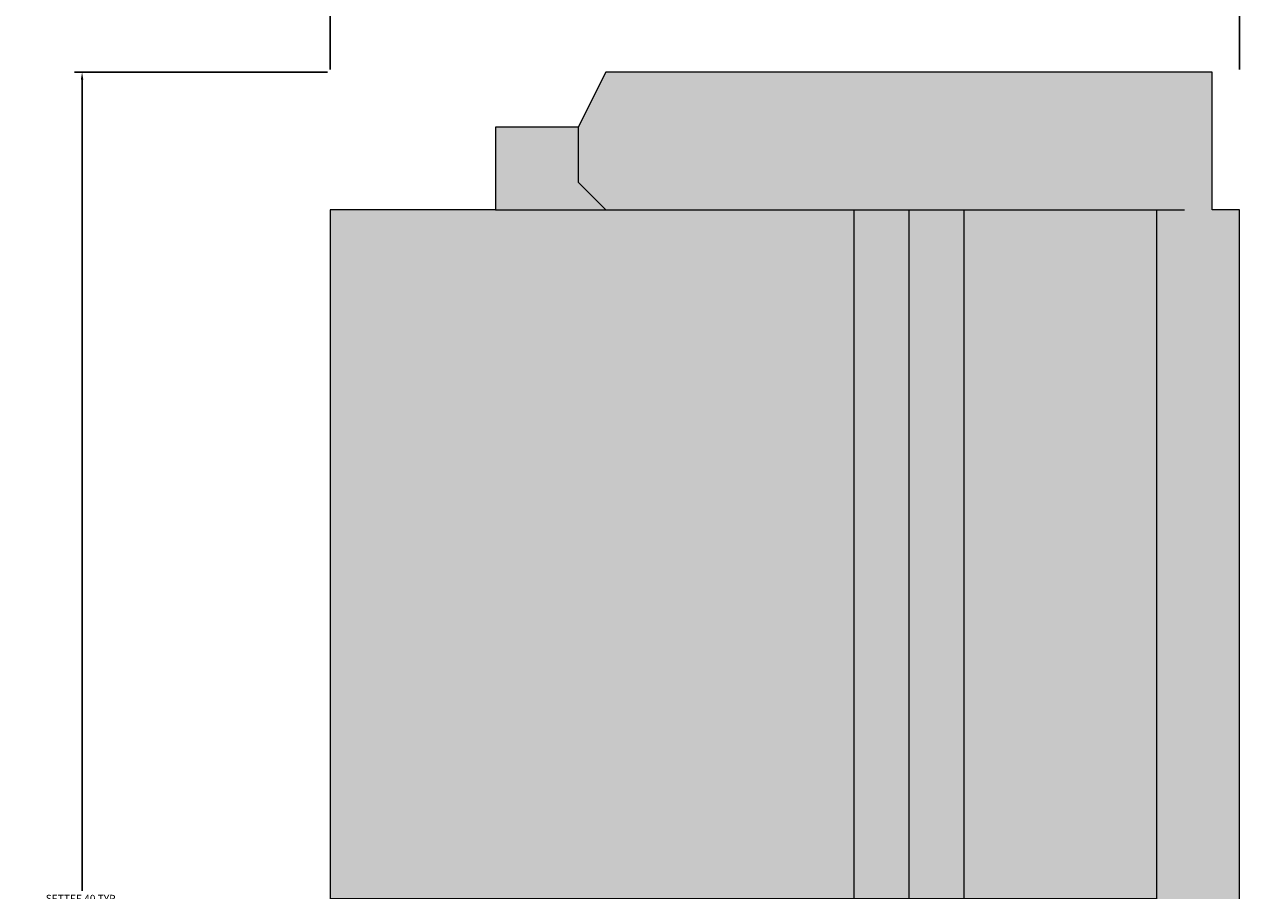
# Model space of a CAD drawing. Units: millimetres. Extents: x 27017497 to 27018854, y 7058029 to 7059154.
# Tile 56 of 91: x 27017980 to 27018010, y 7058348 to 7058369. Entities that reach past the tile are written whole.
import ezdxf

# ---------------------------------------------------------------- set-up
doc = ezdxf.new("R2010")
doc.units = ezdxf.units.MM
doc.layers.add('A-ANNO-DIMS', color=2, linetype='Continuous', lineweight=18)
doc.layers.add('A-FURN', color=8, linetype='Continuous', lineweight=18)
doc.layers.add('A-FURN-PATT', color=177, linetype='Continuous', lineweight=13, true_color=0x293189)
doc.styles.get("Standard").update_dxf_attribs({"font": 'arial.ttf'})
doc.dimstyles.get("Standard").update_dxf_attribs({"dimtxt": 0.18, "dimasz": 0.18, "dimexe": 0.18, "dimexo": 0.0625, "dimgap": 0.09, "dimtad": 0, "dimtih": 1, "dimtoh": 1, "dimdec": 4, "dimzin": 0, "dimdsep": 46, "dimtxsty": 'Standard', "dimcen": 0.09, "dimadec": 0, "dimazin": 0, "dimtfac": 1, "dimtdec": 4, "dimtofl": 0, "dimtmove": 0, "dimatfit": 3, "dimfxl": 1, "dimtolj": 1, "dimtzin": 0, "dimarcsym": 0})

# ---------------------------------------------------------------- blocks, each defined once
blk = doc.blocks.new('SETTEE-TWO-SEAT')
for p, q in [((6.669, 40.014), (6.002, 38.68)), ((21.34, 40.014), (6.669, 40.014)), ((21.34, 36.679), (21.34, 40.014)), ((6.002, 38.68), (4.001, 38.68)), ((4.001, 38.68), (4.001, 36.679)), ((6.002, 38.68), (6.002, 37.346)), ((6.002, 37.346), (6.669, 36.679)), ((0, 36.679), (0, 3.334)), ((4.001, 36.679), (0, 36.679)), ((4.001, 36.679), (6.669, 36.679)), ((6.669, 36.679), (20.673, 36.679)), ((12.671, 36.679), (12.671, 3.334)), ((14.004, 36.679), (14.004, 3.334)), ((15.338, 36.679), (15.338, 3.334)), ((20.006, 3.334), (20.006, 36.679)), ((22.007, 36.679), (21.34, 36.679)), ((22.007, 3.334), (22.007, 36.679)), ((0, 20.007), (20.006, 20.007)), ((0, 3.334), (4.001, 3.334)), ((4.001, 3.334), (6.669, 3.334)), ((4.001, 3.334), (4.001, 1.334)), ((6.002, 2.668), (6.669, 3.334)), ((6.669, 3.334), (20.673, 3.334)), ((21.34, 0), (21.34, 3.334)), ((21.34, 3.334), (22.007, 3.334)), ((6.002, 1.334), (6.002, 2.668)), ((4.001, 1.334), (6.002, 1.334)), ((6.002, 1.334), (6.669, 0)), ((6.669, 0), (21.34, 0))]:
    blk.add_line(p, q)
blk = doc.blocks.new('*D27')
at = {"layer": 'A-ANNO-DIMS', "color": 0, "lineweight": -2, "transparency": 16777216}
for p, q in [((27017987.706, 7058367.587), (27017981.587, 7058367.587)), ((27017981.767, 7058367.407), (27017981.767, 7058347.763)), ((27017981.767, 7058327.753), (27017981.767, 7058347.397)), ((27017987.706, 7058327.573), (27017981.587, 7058327.573))]:
    blk.add_line(p, q, dxfattribs=at)
at = {"layer": 'A-ANNO-DIMS', "color": 0, "transparency": 16777216}
for points in [[(27017981.737, 7058367.407), (27017981.797, 7058367.407), (27017981.767, 7058367.587)], [(27017981.737, 7058327.753), (27017981.797, 7058327.753), (27017981.767, 7058327.573)]]:
    blk.add_solid(points, dxfattribs=at)
at = {"layer": 'Defpoints', "color": 0, "transparency": 16777216}
for p in [(27017981.767, 7058367.587), (27017987.769, 7058367.587), (27017987.769, 7058327.573)]:
    blk.add_point(p, dxfattribs=at)
at = {"layer": 'A-ANNO-DIMS', "color": 0, "transparency": 16777216, "insert": (27017981.767, 7058347.58), "char_height": 0.18, "attachment_point": 5}
blk.add_mtext('\\A1;SETTEE 40 TYP.', dxfattribs=at)
blk = doc.blocks.new('*D28')
at = {"layer": 'A-ANNO-DIMS', "color": 0, "lineweight": -2, "transparency": 16777216}
for p, q in [((27017987.769, 7058367.649), (27017987.769, 7058373.769)), ((27018009.776, 7058367.649), (27018009.776, 7058373.769)), ((27017987.949, 7058373.589), (27017998.243, 7058373.589)), ((27018009.596, 7058373.589), (27017999.302, 7058373.589))]:
    blk.add_line(p, q, dxfattribs=at)
at = {"layer": 'A-ANNO-DIMS', "color": 0, "transparency": 16777216}
for points in [[(27017987.949, 7058373.619), (27017987.949, 7058373.559), (27017987.769, 7058373.589)], [(27018009.596, 7058373.619), (27018009.596, 7058373.559), (27018009.776, 7058373.589)]]:
    blk.add_solid(points, dxfattribs=at)
at = {"layer": 'Defpoints', "color": 0, "transparency": 16777216}
for p in [(27018009.776, 7058373.589), (27017987.769, 7058367.587), (27018009.776, 7058367.587)]:
    blk.add_point(p, dxfattribs=at)
at = {"layer": 'A-ANNO-DIMS', "color": 0, "transparency": 16777216, "insert": (27017998.772, 7058373.589), "char_height": 0.18, "attachment_point": 5}
blk.add_mtext('\\A1;22 TYP.', dxfattribs=at)
blk = doc.blocks.new('*D48')
at = {"layer": 'A-ANNO-DIMS', "color": 0, "lineweight": -2, "transparency": 16777216}
for p, q in [((27018463.498, 7058622.912), (27017497.536, 7058622.912)), ((27017497.716, 7058622.732), (27017497.716, 7058357.753)), ((27017497.716, 7058092.41), (27017497.716, 7058357.389)), ((27018555.129, 7058092.23), (27017497.536, 7058092.23))]:
    blk.add_line(p, q, dxfattribs=at)
at = {"layer": 'A-ANNO-DIMS', "color": 0, "transparency": 16777216}
for points in [[(27017497.686, 7058622.732), (27017497.746, 7058622.732), (27017497.716, 7058622.912)], [(27017497.686, 7058092.41), (27017497.746, 7058092.41), (27017497.716, 7058092.23)]]:
    blk.add_solid(points, dxfattribs=at)
at = {"layer": 'Defpoints', "color": 0, "transparency": 16777216}
for p in [(27018463.561, 7058622.912), (27017497.716, 7058092.23), (27018555.192, 7058092.23)]:
    blk.add_point(p, dxfattribs=at)
at = {"layer": 'A-ANNO-DIMS', "color": 0, "transparency": 16777216, "insert": (27017497.716, 7058357.571), "char_height": 0.18, "attachment_point": 5}
blk.add_mtext('\\A1;530.7', dxfattribs=at)

msp = doc.modelspace()

# ---------------------------------------------------------------- hatches: boundary and pattern name
at = {"layer": 'A-FURN-PATT'}
h = msp.add_hatch(color=256, dxfattribs=at)
h.dxf.hatch_style = 1
h.paths.add_polyline_path([(27017921.559, 7058320.14), (27017906.276, 7058320.14), (27017906.276, 7058304.857), (27017921.559, 7058304.857)])
h.paths.add_polyline_path([(27017921.003, 7058319.584), (27017921.003, 7058305.412), (27017906.831, 7058305.412), (27017906.831, 7058319.584)], flags=16)
h.paths.add_polyline_path([(27017918.811, 7058312.427, -1), (27017909.19, 7058312.427, -1)], flags=0)
h.paths.add_polyline_path([(27017919.33, 7058326.783), (27017919.33, 7058328.117), (27017918.663, 7058328.784), (27017905.325, 7058328.784), (27017905.325, 7058362.129), (27017918.663, 7058362.129), (27017919.33, 7058362.796), (27017919.33, 7058364.13), (27017918.663, 7058365.463), (27017903.991, 7058365.463), (27017903.991, 7058362.129), (27017903.325, 7058362.129), (27017903.325, 7058328.784), (27017903.991, 7058328.784), (27017903.991, 7058325.45), (27017918.663, 7058325.45)])
h.paths.add_polyline_path([(27017925.332, 7058345.456), (27017912.661, 7058345.456), (27017912.661, 7058328.784), (27017918.663, 7058328.784), (27017921.331, 7058328.784), (27017925.332, 7058328.784)])
h.paths.add_polyline_path([(27017925.332, 7058362.129), (27017921.331, 7058362.129), (27017918.663, 7058362.129), (27017912.661, 7058362.129), (27017912.661, 7058345.456), (27017925.332, 7058345.456)])
h.paths.add_polyline_path([(27017909.993, 7058362.129), (27017905.325, 7058362.129), (27017905.325, 7058345.456), (27017909.993, 7058345.456)], flags=17)
h.paths.add_polyline_path([(27017909.993, 7058345.456), (27017905.325, 7058345.456), (27017905.325, 7058328.784), (27017909.993, 7058328.784)], flags=17)
h.paths.add_polyline_path([(27017911.327, 7058345.456), (27017909.993, 7058345.456), (27017909.993, 7058328.784), (27017911.327, 7058328.784)], flags=17)
h.paths.add_polyline_path([(27017912.661, 7058345.456), (27017911.327, 7058345.456), (27017911.327, 7058328.784), (27017912.661, 7058328.784)], flags=17)
h.paths.add_polyline_path([(27017912.661, 7058362.129), (27017911.327, 7058362.129), (27017911.327, 7058345.456), (27017912.661, 7058345.456)], flags=17)
h.paths.add_polyline_path([(27017911.327, 7058362.129), (27017909.993, 7058362.129), (27017909.993, 7058345.456), (27017911.327, 7058345.456)], flags=17)
h.paths.add_polyline_path([(27017973.504, 7058350.536), (27017940.159, 7058350.536), (27017940.159, 7058333.863), (27017973.504, 7058333.863)])
h.paths.add_polyline_path([(27017972.67, 7058349.702), (27017972.67, 7058334.697), (27017940.993, 7058334.697), (27017940.993, 7058349.702)], flags=16)
h.paths.add_polyline_path([(27018000.44, 7058364.252), (27017994.438, 7058364.252), (27017991.77, 7058364.252), (27017987.769, 7058364.252), (27017987.769, 7058347.58), (27018000.44, 7058347.58)])
h.paths.add_polyline_path([(27018000.44, 7058347.58), (27017987.769, 7058347.58), (27017987.769, 7058330.907), (27017991.77, 7058330.907), (27017994.438, 7058330.907), (27018000.44, 7058330.907)])
h.paths.add_polyline_path([(27018009.109, 7058330.907), (27018009.776, 7058330.907), (27018009.776, 7058364.252), (27018009.109, 7058364.252), (27018009.109, 7058367.587), (27017994.438, 7058367.587), (27017993.771, 7058366.253), (27017993.771, 7058364.919), (27017994.438, 7058364.252), (27018007.775, 7058364.252), (27018007.775, 7058330.907), (27017994.438, 7058330.907), (27017993.771, 7058330.241), (27017993.771, 7058328.907), (27017994.438, 7058327.573), (27018009.109, 7058327.573)])
h.paths.add_polyline_path([(27017994.438, 7058330.907), (27017991.77, 7058330.907), (27017991.77, 7058328.907), (27017993.771, 7058328.907), (27017993.771, 7058330.241)])
h.paths.add_polyline_path([(27017993.771, 7058366.253), (27017991.77, 7058366.253), (27017991.77, 7058364.252), (27017994.438, 7058364.252), (27017993.771, 7058364.919)])
h.paths.add_polyline_path([(27018007.775, 7058364.252), (27018003.107, 7058364.252), (27018003.107, 7058347.58), (27018007.775, 7058347.58)], flags=17)
h.paths.add_polyline_path([(27018007.775, 7058347.58), (27018003.107, 7058347.58), (27018003.107, 7058330.907), (27018007.775, 7058330.907)], flags=17)
h.paths.add_polyline_path([(27018003.107, 7058364.252), (27018001.773, 7058364.252), (27018001.773, 7058347.58), (27018003.107, 7058347.58)], flags=17)
h.paths.add_polyline_path([(27018003.107, 7058347.58), (27018001.773, 7058347.58), (27018001.773, 7058330.907), (27018003.107, 7058330.907)], flags=17)
h.paths.add_polyline_path([(27018001.773, 7058347.58), (27018000.44, 7058347.58), (27018000.44, 7058330.907), (27018001.773, 7058330.907)], flags=17)
h.paths.add_polyline_path([(27018001.773, 7058364.252), (27018000.44, 7058364.252), (27018000.44, 7058347.58), (27018001.773, 7058347.58)], flags=17)

# ---------------------------------------------------------------- block references
at = {"layer": 'A-FURN'}
msp.add_blockref('SETTEE-TWO-SEAT', (27017987.769, 7058327.573), dxfattribs=at)

# ---------------------------------------------------------------- dimensions: what is measured, and where the dimension line sits
at = {"layer": 'A-ANNO-DIMS'}
dim = msp.add_linear_dim(base=(27017497.716, 7058092.23), p1=(27018463.561, 7058622.912), p2=(27018555.192, 7058092.23), angle=90, dimstyle='Standard', override={"dimdec": 1, "dimlfac": 1, "dimrnd": 0, "dimzin": 0, "dimdsep": 46, "dimlunit": 2}, dxfattribs=at)
dim.commit()
dim.dimension.update_dxf_attribs({"geometry": '*D48', "text_midpoint": (27017497.716, 7058357.571)})
dim = msp.add_linear_dim(base=(27018009.776, 7058373.589), p1=(27017987.769, 7058367.587), p2=(27018009.776, 7058367.587), text='<> TYP.', dimstyle='Standard', override={"dimdec": 0, "dimlfac": 1, "dimrnd": 0, "dimzin": 0, "dimdsep": 46, "dimlunit": 2}, dxfattribs=at)
dim.commit()
dim.dimension.update_dxf_attribs({"geometry": '*D28', "text_midpoint": (27017998.772, 7058373.589)})
dim = msp.add_linear_dim(base=(27017981.767, 7058367.587), p1=(27017987.769, 7058327.573), p2=(27017987.769, 7058367.587), angle=90, text='SETTEE <> TYP.', dimstyle='Standard', override={"dimdec": 0, "dimlfac": 1, "dimrnd": 0, "dimzin": 0, "dimdsep": 46, "dimlunit": 2}, dxfattribs=at)
dim.commit()
dim.dimension.update_dxf_attribs({"geometry": '*D27', "text_midpoint": (27017981.767, 7058347.58)})

doc.saveas('drawing.dxf')
